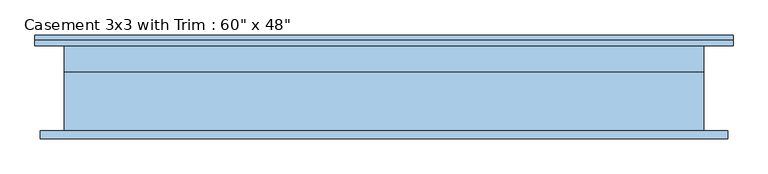
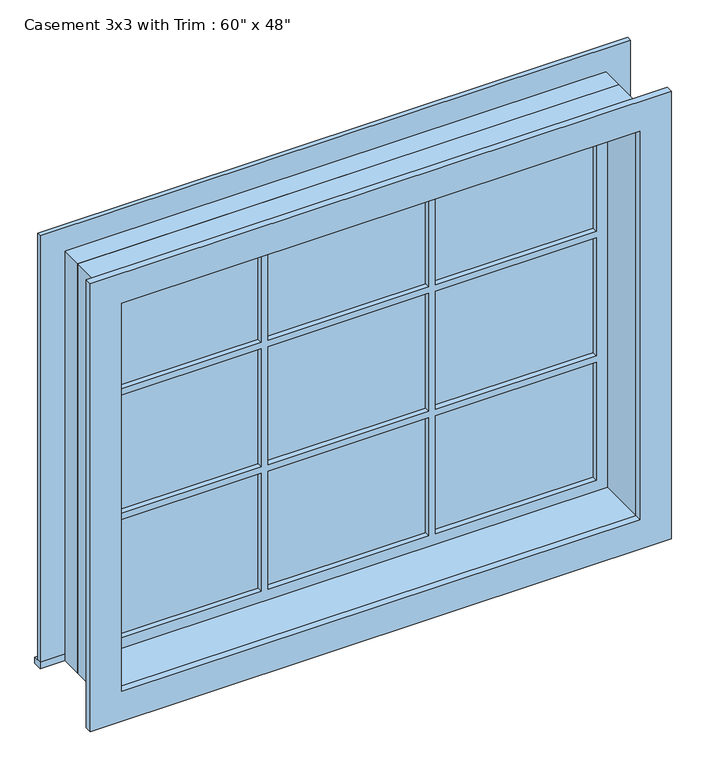
"""IFC4 building model written with IfcOpenShell, lengths in millimetres: window geometry."""

from ifc_helpers import new_model, si_unit, frame, origin, place, context, project, spatial, polyline, outline, extrude, source, transform, mapped, element, save


def window_a4fe791f(model_context):
    return source(origin(), model_context, "Body", "SweptSolid", [
        extrude(outline(polyline([(-831.85, 127.0), (831.85, 127.0), (831.85, 101.6), (-831.85, 101.6), (-831.85, 127.0)])), frame((0.0, 0.0, 914.4), z_axis=(0.0, 0.0, 1.0), x_axis=(1.0, 0.0, 0.0)), (0.0, 0.0, 1.0), 19.05),
        extrude(outline(polyline([(2114.55, -742.95), (2114.55, 742.95), (933.45, 742.95), (933.45, 831.85), (2203.45, 831.85), (2203.45, -831.85), (933.45, -831.85), (933.45, -742.95), (2114.55, -742.95)])), frame((0.0, 101.6, 0.0), z_axis=(0.0, 1.0, 0.0), x_axis=(0.0, 0.0, 1.0)), (0.0, 0.0, 1.0), 12.7),
        extrude(outline(polyline([(245.5333333, 66.675), (698.5, 66.675), (698.5, 53.975), (245.5333333, 53.975), (245.5333333, 66.675)])), frame((0.0, 0.0, 1718.7333333), z_axis=(0.0, 0.0, 1.0), x_axis=(1.0, 0.0, 0.0)), (0.0, 0.0, 1.0), 351.3666667),
        extrude(outline(polyline([(-226.4833333, 66.675), (226.4833333, 66.675), (226.4833333, 53.975), (-226.4833333, 53.975), (-226.4833333, 66.675)])), frame((0.0, 0.0, 1718.7333333), z_axis=(0.0, 0.0, 1.0), x_axis=(1.0, 0.0, 0.0)), (0.0, 0.0, 1.0), 351.3666667),
        extrude(outline(polyline([(-698.5, 66.675), (-245.5333333, 66.675), (-245.5333333, 53.975), (-698.5, 53.975), (-698.5, 66.675)])), frame((0.0, 0.0, 1718.7333333), z_axis=(0.0, 0.0, 1.0), x_axis=(1.0, 0.0, 0.0)), (0.0, 0.0, 1.0), 351.3666667),
        extrude(outline(polyline([(-698.5, 66.675), (-245.5333333, 66.675), (-245.5333333, 53.975), (-698.5, 53.975), (-698.5, 66.675)])), frame((0.0, 0.0, 1348.3166667), z_axis=(0.0, 0.0, 1.0), x_axis=(1.0, 0.0, 0.0)), (0.0, 0.0, 1.0), 351.3666667),
        extrude(outline(polyline([(-226.4833333, 66.675), (226.4833333, 66.675), (226.4833333, 53.975), (-226.4833333, 53.975), (-226.4833333, 66.675)])), frame((0.0, 0.0, 1348.3166667), z_axis=(0.0, 0.0, 1.0), x_axis=(1.0, 0.0, 0.0)), (0.0, 0.0, 1.0), 351.3666667),
        extrude(outline(polyline([(245.5333333, 66.675), (698.5, 66.675), (698.5, 53.975), (245.5333333, 53.975), (245.5333333, 66.675)])), frame((0.0, 0.0, 1348.3166667), z_axis=(0.0, 0.0, 1.0), x_axis=(1.0, 0.0, 0.0)), (0.0, 0.0, 1.0), 351.3666667),
        extrude(outline(polyline([(245.5333333, 66.675), (698.5, 66.675), (698.5, 53.975), (245.5333333, 53.975), (245.5333333, 66.675)])), frame((0.0, 0.0, 977.9), z_axis=(0.0, 0.0, 1.0), x_axis=(1.0, 0.0, 0.0)), (0.0, 0.0, 1.0), 351.3666667),
        extrude(outline(polyline([(-226.4833333, 66.675), (226.4833333, 66.675), (226.4833333, 53.975), (-226.4833333, 53.975), (-226.4833333, 66.675)])), frame((0.0, 0.0, 977.9), z_axis=(0.0, 0.0, 1.0), x_axis=(1.0, 0.0, 0.0)), (0.0, 0.0, 1.0), 351.3666667),
        extrude(outline(polyline([(-698.5, 66.675), (-245.5333333, 66.675), (-245.5333333, 53.975), (-698.5, 53.975), (-698.5, 66.675)])), frame((0.0, 0.0, 977.9), z_axis=(0.0, 0.0, 1.0), x_axis=(1.0, 0.0, 0.0)), (0.0, 0.0, 1.0), 351.3666667),
        extrude(outline(polyline([(2190.75, 819.15), (2190.75, -819.15), (857.25, -819.15), (857.25, 819.15), (2190.75, 819.15)]), holes=[polyline([(2101.85, 730.25), (946.15, 730.25), (946.15, -730.25), (2101.85, -730.25), (2101.85, 730.25)])]), frame((0.0, -120.65, 0.0), z_axis=(0.0, 1.0, 0.0), x_axis=(0.0, 0.0, 1.0)), (0.0, 0.0, 1.0), 19.05),
        extrude(outline(polyline([(2114.55, -742.95), (933.45, -742.95), (933.45, 742.95), (2114.55, 742.95), (2114.55, -742.95)]), holes=[polyline([(2070.1, -245.5333333), (1718.7333333, -245.5333333), (1718.7333333, -698.5), (2070.1, -698.5), (2070.1, -245.5333333)]), polyline([(1699.6833333, -245.5333333), (1348.3166667, -245.5333333), (1348.3166667, -698.5), (1699.6833333, -698.5), (1699.6833333, -245.5333333)]), polyline([(1329.2666667, -245.5333333), (977.9, -245.5333333), (977.9, -698.5), (1329.2666667, -698.5), (1329.2666667, -245.5333333)]), polyline([(2070.1, 226.4833333), (1718.7333333, 226.4833333), (1718.7333333, -226.4833333), (2070.1, -226.4833333), (2070.1, 226.4833333)]), polyline([(1699.6833333, 226.4833333), (1348.3166667, 226.4833333), (1348.3166667, -226.4833333), (1699.6833333, -226.4833333), (1699.6833333, 226.4833333)]), polyline([(1329.2666667, 226.4833333), (977.9, 226.4833333), (977.9, -226.4833333), (1329.2666667, -226.4833333), (1329.2666667, 226.4833333)]), polyline([(2070.1, 698.5), (1718.7333333, 698.5), (1718.7333333, 245.5333333), (2070.1, 245.5333333), (2070.1, 698.5)]), polyline([(1699.6833333, 698.5), (1348.3166667, 698.5), (1348.3166667, 245.5333333), (1699.6833333, 245.5333333), (1699.6833333, 698.5)]), polyline([(1329.2666667, 698.5), (977.9, 698.5), (977.9, 245.5333333), (1329.2666667, 245.5333333), (1329.2666667, 698.5)])]), frame((0.0, 38.1, 0.0), z_axis=(0.0, 1.0, 0.0), x_axis=(0.0, 0.0, 1.0)), (0.0, 0.0, 1.0), 44.45),
        extrude(outline(polyline([(2133.6, -762.0), (914.4, -762.0), (914.4, 762.0), (2133.6, 762.0), (2133.6, -762.0)]), holes=[polyline([(2101.85, -730.25), (2101.85, 730.25), (946.15, 730.25), (946.15, -730.25), (2101.85, -730.25)])]), frame((0.0, -101.6, 0.0), z_axis=(0.0, 1.0, 0.0), x_axis=(0.0, 0.0, 1.0)), (0.0, 0.0, 1.0), 139.7),
        extrude(outline(polyline([(2133.6, 762.0), (2133.6, -762.0), (914.4, -762.0), (914.4, 762.0), (2133.6, 762.0)]), holes=[polyline([(2114.55, 742.95), (933.45, 742.95), (933.45, -742.95), (2114.55, -742.95), (2114.55, 742.95)])]), frame((0.0, 38.1, 0.0), z_axis=(0.0, 1.0, 0.0), x_axis=(0.0, 0.0, 1.0)), (0.0, 0.0, 1.0), 63.5),
    ])


if __name__ == "__main__":
    model = new_model("IFC4")
    model_context = context("Model", 3, world=origin())
    ifc_project = project(units=[si_unit("LENGTHUNIT", "METRE", prefix="MILLI")], contexts=[model_context])
    site = spatial("IfcSite", under=ifc_project)
    building = spatial("IfcBuilding", under=site)
    placement = place(None, origin())
    window_shape = window_a4fe791f(model_context)
    element("IfcWindow", 1, ObjectType="Casement 3x3 with Trim : 60\" x 48\"", at=placement, inside=building, context=model_context, shape_type="MappedRepresentation", body=[
        mapped(window_shape, transform((0.0, 0.0, 0.0), x_axis=(1.0, 0.0, 0.0), y_axis=(0.0, 1.0, 0.0), z_axis=(0.0, 0.0, 1.0))),
    ])
    save(model, "model.ifc")

# Revit data of these elements
# Type "Casement 3x3 with Trim : 60\" x 48\""
#   Type Mark = "10"
#   Construction Type Id = "GSP4R"
#   Assembly Code = "B2020100"
#   Analytic Construction = "1/8 in Pilkington single glazing"
#   Visual Light Transmittance = 0.9
#   Solar Heat Gain Coefficient = 0.78
#   Heat Transfer Coefficient (U) = 0.6496 BTU/(h·ft²·°F)
#   Height = 4' - 0"
#   Default Sill Height = 3' - 0"
#   Trim Projection - Ext. = 0' - 0 1/2"
#   Trim Projection - Int. = 0' - 0 3/4"
#   Trim Width - Exterior = 0' - 3 1/2"
#   Trim Width - Interior = 0' - 3 1/2"
#   Width = 5' - 0"
#   Window Inset = 0' - 0 3/4"
#   Define Thermal Properties by = 1
#   Glass Pane Material = Glass
#   Sash Material = Sash
#   Trim Exterior Material = Trim
#   Trim Interior Material = Trim
#   Wall Closure = (empty or 0)
# Element 1 (IfcWindow, "Casement 3x3 with Trim : 60\" x 48\"")
#   Materials on its faces: "Sash", "Glass", "Trim"
# Materials
#   "Glass": class "Glass", colour RGB 0 128 192, transparency 0.75, Description = "Soda Lime Glass", Cost = 0
#   "Sash": class "Wood", colour RGB 224 178 126, transparency 0
#   "Trim": class "Wood", colour RGB 224 178 126, transparency 0
